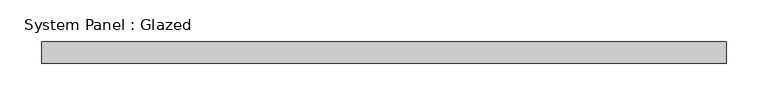
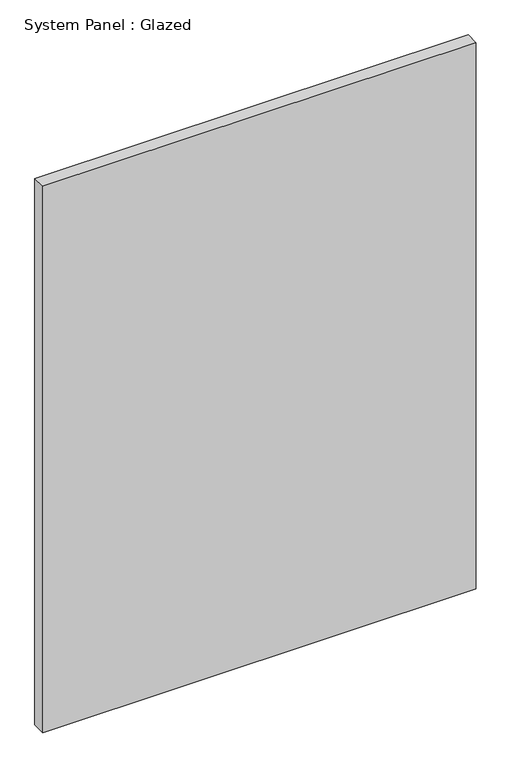
"""IFC4 building model written with IfcOpenShell, lengths in millimetres: plate geometry, System Panel : Glazed."""

from ifc_helpers import new_model, si_unit, origin, origin_with_axes, place, context, project, spatial, polyline, outline, extrude, source, transform, mapped, element, save


def system_panel_glazed_d6173012(model_context):
    return source(origin(), model_context, "Body", "SweptSolid", [
        extrude(outline(polyline([(409.575, 19.05), (-409.575, 19.05), (-409.575, 44.45), (409.575, 44.45), (409.575, 19.05)])), origin_with_axes(), (0.0, 0.0, 1.0), 1092.2),
    ])


if __name__ == "__main__":
    model = new_model("IFC4")
    model_context = context("Model", 3, world=origin())
    ifc_project = project(units=[si_unit("LENGTHUNIT", "METRE", prefix="MILLI")], contexts=[model_context])
    site = spatial("IfcSite", under=ifc_project)
    building = spatial("IfcBuilding", under=site)
    placement = place(None, origin())
    system_panel_glazed_shape = system_panel_glazed_d6173012(model_context)
    element("IfcPlate", 1, ObjectType="System Panel : Glazed", at=placement, inside=building, context=model_context, shape_type="MappedRepresentation", body=[
        mapped(system_panel_glazed_shape, transform((0.0, 0.0, 0.0), x_axis=(1.0, 0.0, 0.0), y_axis=(0.0, 1.0, 0.0), z_axis=(0.0, 0.0, 1.0))),
    ])
    save(model, "model.ifc")

# Revit data of these elements
# Type "System Panel : Glazed"
#   Construction Type Id = "GSP4R"
#   Analytic Construction = "1/8 in Pilkington single glazing"
#   Visual Light Transmittance = 0.9
#   Solar Heat Gain Coefficient = 0.86
#   Heat Transfer Coefficient (U) = 1.18115 BTU/(h·ft²·°F)
#   Define Thermal Properties by = 1
# Element 1 (IfcPlate, "System Panel : Glazed")
#   Materials on its faces: "Glass"
# Materials
#   "Glass": class "Glass", colour RGB 0 128 192, transparency 0.75, Description = "Soda Lime Glass", Cost = 0
